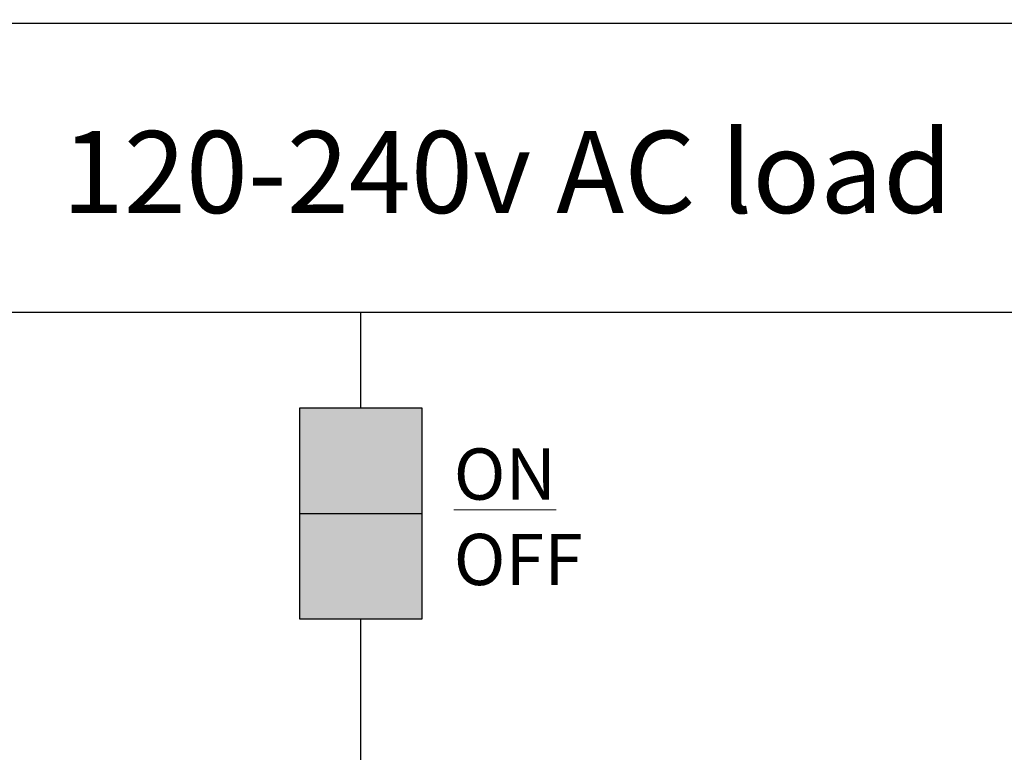
# Model space of a CAD drawing. Units: millimetres. Extents: x -8 to 285, y 5 to 221.
# Tile 27 of 30: x 172 to 221, y 185 to 221. Entities that reach past the tile are written whole.
import ezdxf

# ---------------------------------------------------------------- set-up
doc = ezdxf.new("R2010")
doc.units = ezdxf.units.MM
for name, color, linetype, lineweight in [('A-ANNO-DIMS', 2, 'Continuous', 18), ('E-ANNO-TEXT', 7, 'Continuous', 18), ('E-EQPM-PATT', 252, 'Continuous', 13), ('E-LITE-SWCH', 7, 'Continuous', 25)]:
    doc.layers.add(name, color=color, linetype=linetype, lineweight=lineweight)
doc.layers.add('E-POWR-AC-LINE', color=30, linetype='Continuous', lineweight=25, true_color=0xf26722)
doc.styles.get("Standard").update_dxf_attribs({"font": 'arial.ttf'})
doc.dimstyles.get("Standard").update_dxf_attribs({"dimtxt": 0.18, "dimasz": 0.18, "dimexe": 0.18, "dimexo": 0.0625, "dimgap": 0.09, "dimtad": 0, "dimtih": 1, "dimtoh": 1, "dimdec": 4, "dimzin": 0, "dimdsep": 46, "dimtxsty": 'Standard', "dimcen": 0.09, "dimadec": 0, "dimazin": 0, "dimtfac": 1, "dimtdec": 4, "dimtofl": 0, "dimtmove": 0, "dimatfit": 3, "dimfxl": 1, "dimtolj": 1, "dimtzin": 0, "dimarcsym": 0})

# ---------------------------------------------------------------- blocks, each defined once
blk = doc.blocks.new('SWITCH-ON-OFF')
blk.add_line((0, 5.151), (5.948, 5.151))
blk.add_lwpolyline([(0, 10.303), (5.948, 10.303), (5.948, 0), (0, 0)], close=True)
blk = doc.blocks.new('*D9')
at = {"layer": 'A-ANNO-DIMS', "color": 0, "lineweight": -2, "transparency": 16777216}
for p, q in [((6.672, 133.79), (6.672, 220.737)), ((6.852, 220.557), (138.33, 220.557)), ((270.739, 220.557), (139.262, 220.557)), ((270.919, 206.519), (270.919, 220.737))]:
    blk.add_line(p, q, dxfattribs=at)
at = {"layer": 'A-ANNO-DIMS', "color": 0, "transparency": 16777216}
for points in [[(6.852, 220.587), (6.852, 220.527), (6.672, 220.557)], [(270.739, 220.587), (270.739, 220.527), (270.919, 220.557)]]:
    blk.add_solid(points, dxfattribs=at)
at = {"layer": 'Defpoints', "color": 0, "transparency": 16777216}
for p in [(270.919, 220.557), (270.919, 206.457), (6.672, 133.727)]:
    blk.add_point(p, dxfattribs=at)
at = {"layer": 'A-ANNO-DIMS', "color": 0, "transparency": 16777216, "insert": (138.796, 220.557), "char_height": 0.18, "attachment_point": 5}
blk.add_mtext('\\A1;264.25', dxfattribs=at)

msp = doc.modelspace()

# ---------------------------------------------------------------- hatches: boundary and pattern name
at = {"layer": 'E-EQPM-PATT'}
h = msp.add_hatch(color=256, dxfattribs=at)
h.set_gradient(color2=(0, 0, 0), tint=1)
h.paths.add_polyline_path([(41.1717, 67.9064, 1), (39.1717, 67.9064, 1)])
h.paths.add_polyline_path([(47.1717, 67.9064, 1), (45.1717, 67.9064, 1)])
h.paths.add_polyline_path([(53.1717, 67.9064, 1), (51.1717, 67.9064, 1)])
h.paths.add_polyline_path([(57.1717, 67.9064, 1), (59.1717, 67.9064, 1)])
h.paths.add_polyline_path([(65.1717, 67.9064, 1), (63.1717, 67.9064, 1)])
h.paths.add_polyline_path([(69.1717, 67.9064, 1), (71.1717, 67.9064, 1)])
h.paths.add_polyline_path([(148.1394, 196.6424), (148.1394, 201.7939), (142.1909, 201.7939), (142.1909, 196.6424)])
h.paths.add_polyline_path([(186.1388, 201.7939), (186.1388, 196.6424), (192.0873, 196.6424), (192.0873, 201.7939)])
h.paths.add_polyline_path([(234.0155, 196.6424), (234.0155, 201.7939), (228.067, 201.7939), (228.067, 196.6424)])
h = msp.add_hatch(color=256, dxfattribs=at)
h.set_gradient(color1=(254, 234, 185), color2=(254, 234, 185), tint=1)
h.paths.add_polyline_path([(148.1394, 191.4908), (148.1394, 196.6424), (142.1909, 196.6424), (142.1909, 191.4908)])
h.paths.add_polyline_path([(186.1388, 191.4908), (192.0873, 191.4908), (192.0873, 196.6424), (186.1388, 196.6424)])
h.paths.add_polyline_path([(228.067, 191.4908), (234.0155, 191.4908), (234.0155, 196.6424), (228.067, 196.6424)])

# ---------------------------------------------------------------- linework, layer by layer
at = {"layer": 'E-POWR-AC-LINE'}
for p, q in [((189.1131, 201.7939), (189.1131, 206.4568)), ((189.1131, 184.1071), (189.1131, 191.4908))]:
    msp.add_line(p, q, dxfattribs=at)
msp.add_lwpolyline([(244.6186, 34.6512), (244.6186, 49.925), (270.9192, 49.925), (270.9192, 206.4568), (145.1651, 206.4568), (145.1651, 201.7939)], dxfattribs=at)

# ---------------------------------------------------------------- block references
at = {"layer": 'E-LITE-SWCH'}
msp.add_blockref('SWITCH-ON-OFF', (186.1389, 191.491), dxfattribs=at)

# ---------------------------------------------------------------- texts
at = {"layer": 'E-ANNO-TEXT', "attachment_point": 1}
for s, width, heights, insert, char_height in [('120-240v AC load', 65.111825, [0], (174.5145, 215.3049), 4), (' {\\LON\\P} OFF', 8.619646, [7.2553], (192.8785, 199.8179), 2.5)]:
    msp.add_mtext_dynamic_manual_height_columns(s, width=width, gutter_width=12.5, heights=heights, dxfattribs=dict(at, insert=insert, char_height=char_height))

# ---------------------------------------------------------------- dimensions: what is measured, and where the dimension line sits
at = {"layer": 'A-ANNO-DIMS'}
dim = msp.add_linear_dim(base=(270.9192, 220.5568), p1=(6.6725, 133.7273), p2=(270.9192, 206.4568), dimstyle='Standard', override={"dimdec": 2, "dimlfac": 1, "dimrnd": 0, "dimzin": 0, "dimdsep": 46, "dimlunit": 2}, dxfattribs=at)
dim.commit()
dim.dimension.update_dxf_attribs({"geometry": '*D9', "text_midpoint": (138.7958, 220.5568)})

doc.saveas('drawing.dxf')
